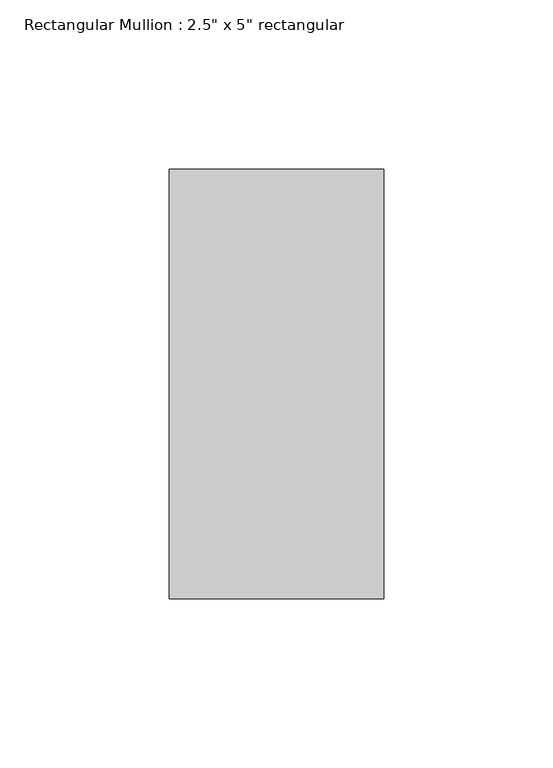
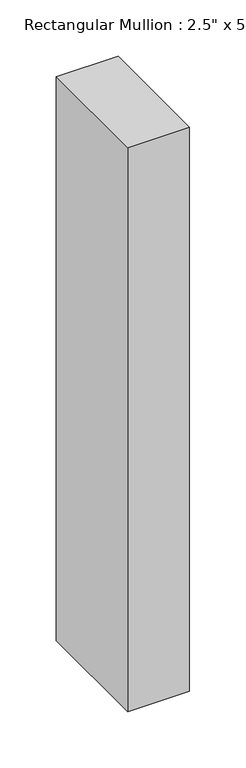
"""IFC4 building model written with IfcOpenShell, lengths in millimetres: member geometry."""

from ifc_helpers import new_model, si_unit, frame, origin, place, context, project, spatial, polyline, outline, extrude, source, transform, mapped, element, save


def member_b864958b(model_context):
    return source(origin(), model_context, "Body", "SweptSolid", [
        extrude(outline(polyline([(0.0, 63.5), (0.0, -63.5), (-63.5, -63.5), (-63.5, 63.5), (0.0, 63.5)])), frame((0.0, 0.0, -612.7937999), z_axis=(0.0, 0.0, 1.0), x_axis=(1.0, 0.0, 0.0)), (0.0, 0.0, 1.0), 612.7937999),
    ])


if __name__ == "__main__":
    model = new_model("IFC4")
    model_context = context("Model", 3, world=origin())
    ifc_project = project(units=[si_unit("LENGTHUNIT", "METRE", prefix="MILLI")], contexts=[model_context])
    site = spatial("IfcSite", under=ifc_project)
    building = spatial("IfcBuilding", under=site)
    placement = place(None, origin())
    member_shape = member_b864958b(model_context)
    element("IfcMember", 1, ObjectType="Rectangular Mullion : 2.5\" x 5\" rectangular", at=placement, inside=building, context=model_context, shape_type="MappedRepresentation", body=[
        mapped(member_shape, transform((0.0, 0.0, 0.0), x_axis=(1.0, 0.0, 0.0), y_axis=(0.0, 1.0, 0.0), z_axis=(0.0, 0.0, 1.0))),
    ])
    save(model, "model.ifc")

# Revit data of these elements
# Type "Rectangular Mullion : 2.5\" x 5\" rectangular"
#   built-in parameter 1007304 = 0.416667 (stored number, unit not read)
#   built-in parameter 1007301 = 0.104167 (stored number, unit not read)
#   built-in parameter 1007300 = 0.104167 (stored number, unit not read)
# Element 1 (IfcMember, "Rectangular Mullion : 2.5\" x 5\" rectangular")
#   Materials on its faces: "Aluminum"
# Materials
#   "Aluminum": class "Metal", colour RGB 247 247 247, transparency 0, Description = "Aluminum 6061", Cost = 0
